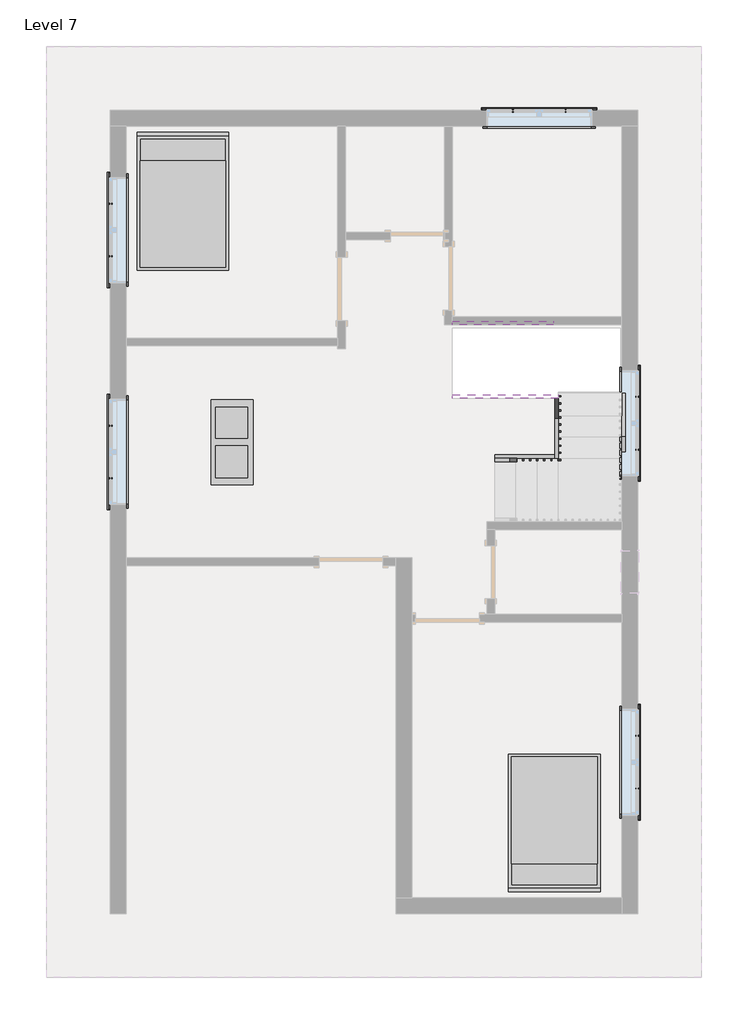
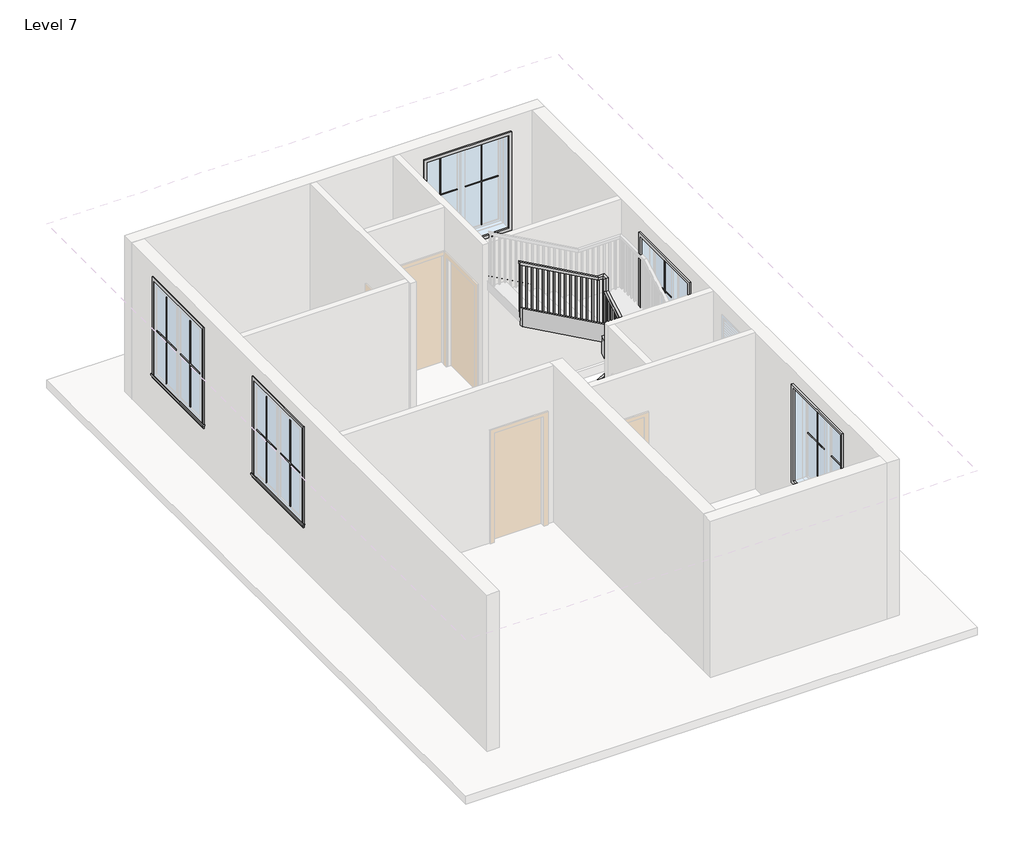
# One storey, part 2 of 2: 21 proxies, 6 members, 2 furniture elements, 1 railing.
"""IFC4 building model written with IfcOpenShell, lengths in millimetres."""

from ifc_helpers import new_model, si_unit, frame, origin, place, context, project, spatial, polyline, outline, extrude, faceted_brep, transform, mapped, element, save
from components import muntin_pattern_2x2_muntin_pattern_2x2_f6a80940, muntin_pattern_2x2_muntin_pattern_2x2_09b00a1c, trim_window_exterior_flat_with_sill_698ed857, trim_window_interior_flat_picture_frame_92551a5e, coffee_table_with_brass_mullions_11320_coffee_table_with_5962bef7, bed_17739_bed_17739_15c61121

model = new_model("IFC4")

# Units and contexts
model_context = context("Model", 3, world=origin())
ifc_project = project(units=[si_unit("LENGTHUNIT", "METRE", prefix="MILLI")], contexts=[model_context])

# Site, building, storey
site = spatial("IfcSite", under=ifc_project)
building = spatial("IfcBuilding", under=site)
storey = spatial("IfcBuildingStorey", under=building, Name="Level 7", Elevation=16002.0)

# Proxies
placement = place(None, origin())
muntin_pattern_2x2_muntin_pattern_2x2_shape = muntin_pattern_2x2_muntin_pattern_2x2_f6a80940(model_context)
element("IfcBuildingElementProxy", 1, Name="Muntin Pattern_2x2 : Muntin Pattern_2x2", ObjectType="Muntin Pattern_2x2 : Muntin Pattern_2x2", at=placement, inside=storey, context=model_context, shape_type="MappedRepresentation", body=[
    mapped(muntin_pattern_2x2_muntin_pattern_2x2_shape, transform((-4589.1575206, 441.8004493, 16986.25), x_axis=(0.0, 1.0, 0.0), y_axis=(-1.0, 0.0, 0.0), z_axis=(0.0, 0.0, 1.0))),
])
element("IfcBuildingElementProxy", 2, Name="Muntin Pattern_2x2 : Muntin Pattern_2x2", ObjectType="Muntin Pattern_2x2 : Muntin Pattern_2x2", at=placement, inside=storey, context=model_context, shape_type="MappedRepresentation", body=[
    mapped(muntin_pattern_2x2_muntin_pattern_2x2_shape, transform((-4589.1575206, 3632.6754493, 16986.25), x_axis=(0.0, 1.0, 0.0), y_axis=(-1.0, 0.0, 0.0), z_axis=(0.0, 0.0, 1.0))),
])
element("IfcBuildingElementProxy", 3, Name="Muntin Pattern_2x2 : Muntin Pattern_2x2", ObjectType="Muntin Pattern_2x2 : Muntin Pattern_2x2", at=placement, inside=storey, context=model_context, shape_type="MappedRepresentation", body=[
    mapped(muntin_pattern_2x2_muntin_pattern_2x2_shape, transform((1197.2799794, 5726.5879493, 16986.25), x_axis=(1.0, 0.0, 0.0), y_axis=(0.0, 1.0, 0.0), z_axis=(0.0, 0.0, 1.0))),
])
element("IfcBuildingElementProxy", 4, Name="Muntin Pattern_2x2 : Muntin Pattern_2x2", ObjectType="Muntin Pattern_2x2 : Muntin Pattern_2x2", at=placement, inside=storey, context=model_context, shape_type="MappedRepresentation", body=[
    mapped(muntin_pattern_2x2_muntin_pattern_2x2_shape, transform((2986.3924794, 1613.3754493, 16986.25), x_axis=(0.0, -1.0, 0.0), y_axis=(1.0, 0.0, 0.0), z_axis=(0.0, 0.0, 1.0))),
])
element("IfcBuildingElementProxy", 5, Name="Muntin Pattern_2x2 : Muntin Pattern_2x2", ObjectType="Muntin Pattern_2x2 : Muntin Pattern_2x2", at=placement, inside=storey, context=model_context, shape_type="MappedRepresentation", body=[
    mapped(muntin_pattern_2x2_muntin_pattern_2x2_shape, transform((2986.3924794, -3260.2495507, 16986.25), x_axis=(0.0, -1.0, 0.0), y_axis=(1.0, 0.0, 0.0), z_axis=(0.0, 0.0, 1.0))),
])
muntin_pattern_2x2_muntin_pattern_2x2_2_shape = muntin_pattern_2x2_muntin_pattern_2x2_09b00a1c(model_context)
element("IfcBuildingElementProxy", 6, Name="Muntin Pattern_2x2 : Muntin Pattern_2x2", ObjectType="Muntin Pattern_2x2 : Muntin Pattern_2x2", at=placement, inside=storey, context=model_context, shape_type="MappedRepresentation", body=[
    mapped(muntin_pattern_2x2_muntin_pattern_2x2_2_shape, transform((-4589.1575206, 1200.6254493, 16986.25), x_axis=(0.0, -1.0, 0.0), y_axis=(1.0, 0.0, 0.0), z_axis=(0.0, 0.0, 1.0))),
])
element("IfcBuildingElementProxy", 7, Name="Muntin Pattern_2x2 : Muntin Pattern_2x2", ObjectType="Muntin Pattern_2x2 : Muntin Pattern_2x2", at=placement, inside=storey, context=model_context, shape_type="MappedRepresentation", body=[
    mapped(muntin_pattern_2x2_muntin_pattern_2x2_2_shape, transform((-4589.1575206, 4391.5004493, 16986.25), x_axis=(0.0, -1.0, 0.0), y_axis=(1.0, 0.0, 0.0), z_axis=(0.0, 0.0, 1.0))),
])
element("IfcBuildingElementProxy", 8, Name="Muntin Pattern_2x2 : Muntin Pattern_2x2", ObjectType="Muntin Pattern_2x2 : Muntin Pattern_2x2", at=placement, inside=storey, context=model_context, shape_type="MappedRepresentation", body=[
    mapped(muntin_pattern_2x2_muntin_pattern_2x2_2_shape, transform((1956.1049794, 5726.5879493, 16986.25), x_axis=(-1.0, 0.0, 0.0), y_axis=(0.0, -1.0, 0.0), z_axis=(0.0, 0.0, 1.0))),
])
element("IfcBuildingElementProxy", 9, Name="Muntin Pattern_2x2 : Muntin Pattern_2x2", ObjectType="Muntin Pattern_2x2 : Muntin Pattern_2x2", at=placement, inside=storey, context=model_context, shape_type="MappedRepresentation", body=[
    mapped(muntin_pattern_2x2_muntin_pattern_2x2_2_shape, transform((2986.3924794, 854.5504493, 16986.25), x_axis=(0.0, 1.0, 0.0), y_axis=(-1.0, 0.0, 0.0), z_axis=(0.0, 0.0, 1.0))),
])
element("IfcBuildingElementProxy", 10, Name="Muntin Pattern_2x2 : Muntin Pattern_2x2", ObjectType="Muntin Pattern_2x2 : Muntin Pattern_2x2", at=placement, inside=storey, context=model_context, shape_type="MappedRepresentation", body=[
    mapped(muntin_pattern_2x2_muntin_pattern_2x2_2_shape, transform((2986.3924794, -4019.0745507, 16986.25), x_axis=(0.0, 1.0, 0.0), y_axis=(-1.0, 0.0, 0.0), z_axis=(0.0, 0.0, 1.0))),
])
trim_window_exterior_flat_with_sill_shape = trim_window_exterior_flat_with_sill_698ed857(model_context)
element("IfcBuildingElementProxy", 11, Name="Trim-Window-Exterior-Flat : with Sill", ObjectType="Trim-Window-Exterior-Flat : with Sill", at=placement, inside=storey, context=model_context, shape_type="MappedRepresentation", body=[
    mapped(trim_window_exterior_flat_with_sill_shape, transform((-4598.6825206, 821.2129493, 18745.2), x_axis=(0.0, -1.0, 0.0), y_axis=(0.0, 0.0, 1.0), z_axis=(-1.0, 0.0, 0.0))),
])
element("IfcBuildingElementProxy", 12, Name="Trim-Window-Exterior-Flat : with Sill", ObjectType="Trim-Window-Exterior-Flat : with Sill", at=placement, inside=storey, context=model_context, shape_type="MappedRepresentation", body=[
    mapped(trim_window_exterior_flat_with_sill_shape, transform((-4598.6825206, 4012.0879493, 18745.2), x_axis=(0.0, -1.0, 0.0), y_axis=(0.0, 0.0, 1.0), z_axis=(-1.0, 0.0, 0.0))),
])
element("IfcBuildingElementProxy", 13, Name="Trim-Window-Exterior-Flat : with Sill", ObjectType="Trim-Window-Exterior-Flat : with Sill", at=placement, inside=storey, context=model_context, shape_type="MappedRepresentation", body=[
    mapped(trim_window_exterior_flat_with_sill_shape, transform((1576.6924794, 5736.1129493, 18745.2), x_axis=(-1.0, 0.0, 0.0), y_axis=(0.0, 0.0, 1.0), z_axis=(0.0, 1.0, 0.0))),
])
element("IfcBuildingElementProxy", 14, Name="Trim-Window-Exterior-Flat : with Sill", ObjectType="Trim-Window-Exterior-Flat : with Sill", at=placement, inside=storey, context=model_context, shape_type="MappedRepresentation", body=[
    mapped(trim_window_exterior_flat_with_sill_shape, transform((2995.9174794, 1233.9629493, 18745.2), x_axis=(0.0, 1.0, 0.0), y_axis=(0.0, 0.0, 1.0), z_axis=(1.0, 0.0, 0.0))),
])
element("IfcBuildingElementProxy", 15, Name="Trim-Window-Exterior-Flat : with Sill", ObjectType="Trim-Window-Exterior-Flat : with Sill", at=placement, inside=storey, context=model_context, shape_type="MappedRepresentation", body=[
    mapped(trim_window_exterior_flat_with_sill_shape, transform((2995.9174794, -3639.6620507, 18745.2), x_axis=(0.0, 1.0, 0.0), y_axis=(0.0, 0.0, 1.0), z_axis=(1.0, 0.0, 0.0))),
])
trim_window_interior_flat_picture_frame_shape = trim_window_interior_flat_picture_frame_92551a5e(model_context)
element("IfcBuildingElementProxy", 16, Name="Trim-Window-Interior-Flat : Picture Frame", ObjectType="Trim-Window-Interior-Flat : Picture Frame", at=placement, inside=storey, context=model_context, shape_type="MappedRepresentation", body=[
    mapped(trim_window_interior_flat_picture_frame_shape, transform((-4370.0825206, 821.2129493, 18745.2), x_axis=(0.0, 1.0, 0.0), y_axis=(0.0, 0.0, 1.0), z_axis=(1.0, 0.0, 0.0))),
])
element("IfcBuildingElementProxy", 17, Name="Trim-Window-Interior-Flat : Picture Frame", ObjectType="Trim-Window-Interior-Flat : Picture Frame", at=placement, inside=storey, context=model_context, shape_type="MappedRepresentation", body=[
    mapped(trim_window_interior_flat_picture_frame_shape, transform((-4370.0825206, 4012.0879493, 18745.2), x_axis=(0.0, 1.0, 0.0), y_axis=(0.0, 0.0, 1.0), z_axis=(1.0, 0.0, 0.0))),
])
element("IfcBuildingElementProxy", 18, Name="Trim-Window-Interior-Flat : Picture Frame", ObjectType="Trim-Window-Interior-Flat : Picture Frame", at=placement, inside=storey, context=model_context, shape_type="MappedRepresentation", body=[
    mapped(trim_window_interior_flat_picture_frame_shape, transform((1576.6924794, 5507.5129493, 18745.2), x_axis=(1.0, 0.0, 0.0), y_axis=(0.0, 0.0, 1.0), z_axis=(0.0, -1.0, 0.0))),
])
element("IfcBuildingElementProxy", 19, Name="Trim-Window-Interior-Flat : Picture Frame", ObjectType="Trim-Window-Interior-Flat : Picture Frame", at=placement, inside=storey, context=model_context, shape_type="MappedRepresentation", body=[
    mapped(trim_window_interior_flat_picture_frame_shape, transform((2767.3174794, 1233.9629493, 18745.2), x_axis=(0.0, -1.0, 0.0), y_axis=(0.0, 0.0, 1.0), z_axis=(-1.0, 0.0, 0.0))),
])
element("IfcBuildingElementProxy", 20, Name="Trim-Window-Interior-Flat : Picture Frame", ObjectType="Trim-Window-Interior-Flat : Picture Frame", at=placement, inside=storey, context=model_context, shape_type="MappedRepresentation", body=[
    mapped(trim_window_interior_flat_picture_frame_shape, transform((2767.3174794, -3639.6620507, 18745.2), x_axis=(0.0, -1.0, 0.0), y_axis=(0.0, 0.0, 1.0), z_axis=(-1.0, 0.0, 0.0))),
])
coffee_table_with_brass_mullions_11320_coffee_table_with_shape = coffee_table_with_brass_mullions_11320_coffee_table_with_5962bef7(model_context)
element("IfcBuildingElementProxy", 21, Name="coffee_table_with_brass_mullions_11320 : coffee_table_with_brass_mullions_11320", ObjectType="coffee_table_with_brass_mullions_11320 : coffee_table_with_brass_mullions_11320", at=placement, inside=storey, context=model_context, shape_type="MappedRepresentation", body=[
    mapped(coffee_table_with_brass_mullions_11320_coffee_table_with_shape, transform((-2412.0418112, 1596.9678033, 16002.0), x_axis=(0.0, 1.0, 0.0), y_axis=(-1.0, 0.0, 0.0), z_axis=(0.0, 0.0, 1.0))),
])

# Furniture
bed_17739_bed_17739_shape = bed_17739_bed_17739_15c61121(model_context)
element("IfcFurniture", 22, ObjectType="Bed_17739 : Bed_17739", at=placement, inside=storey, context=model_context, shape_type="MappedRepresentation", body=[
    mapped(bed_17739_bed_17739_shape, transform((-3550.9325206, 4402.6129493, 16002.0), x_axis=(1.0, 0.0, 0.0), y_axis=(0.0, 1.0, 0.0), z_axis=(0.0, 0.0, 1.0))),
])
element("IfcFurniture", 23, ObjectType="Bed_17739 : Bed_17739", at=placement, inside=storey, context=model_context, shape_type="MappedRepresentation", body=[
    mapped(bed_17739_bed_17739_shape, transform((1795.7674794, -4487.3870507, 16002.0), x_axis=(-1.0, 0.0, 0.0), y_axis=(0.0, -1.0, 0.0), z_axis=(0.0, 0.0, 1.0))),
])

# Members
element("IfcMember", 24, ObjectType="Stringer - 2\" Width", at=placement, inside=storey, context=model_context, shape_type="SweptSolid", body=[
    extrude(outline(polyline([(16209.5983948, 938.5174794), (16002.0, 938.5174794), (16002.0, 1192.4619822), (16340.6974984, 1802.1174794), (16689.3761726, 1802.1174794), (16209.5983948, 938.5174794)])), frame((0.0, 732.3129493, 0.0), z_axis=(0.0, 1.0, 0.0), x_axis=(0.0, 0.0, 1.0)), (0.0, 0.0, 1.0), 50.8),
])
element("IfcMember", 25, ObjectType="Stringer - 2\" Width", at=placement, inside=storey, context=model_context, shape_type="SweptSolid", body=[
    extrude(outline(polyline([(732.3129493, 16538.253054), (732.3129493, 16886.9317281), (1595.9129493, 17366.7095059), (1595.9129493, 17018.0308318), (732.3129493, 16538.253054)])), frame((1802.1174794, 0.0, 0.0), z_axis=(1.0, 0.0, 0.0), x_axis=(0.0, 1.0, 0.0)), (0.0, 0.0, 1.0), 50.8),
])
element("IfcMember", 26, ObjectType="Stringer - 2\" Width", at=placement, inside=storey, context=model_context, shape_type="SweptSolid", body=[
    extrude(outline(polyline([(17215.5863873, 1852.9174794), (17564.2650614, 1852.9174794), (18410.9317281, 328.9174794), (18062.253054, 328.9174794), (17215.5863873, 1852.9174794)])), frame((0.0, 1595.9129493, 0.0), z_axis=(0.0, 1.0, 0.0), x_axis=(0.0, 0.0, 1.0)), (0.0, 0.0, 1.0), 50.8),
])
element("IfcMember", 27, ObjectType="Stringer - 2\" Width", at=placement, inside=storey, context=model_context, shape_type="SweptSolid", body=[
    extrude(outline(polyline([(16209.5983948, 938.5174794), (16002.0, 938.5174794), (16002.0, 1192.4619822), (16378.9317281, 1870.9390928), (16378.9317281, 1243.3174794), (16209.5983948, 938.5174794)])), frame((0.0, -232.8870507, 0.0), z_axis=(0.0, 1.0, 0.0), x_axis=(0.0, 0.0, 1.0)), (0.0, 0.0, 1.0), 50.8),
])
element("IfcMember", 28, ObjectType="Stringer - 2\" Width", at=placement, inside=storey, context=model_context, shape_type="SweptSolid", body=[
    extrude(outline(polyline([(714.2913359, 16876.9197207), (1037.1129493, 17056.2650614), (1664.7345627, 17056.2650614), (1341.9129493, 16876.9197207), (714.2913359, 16876.9197207)])), frame((2767.3174794, 0.0, 0.0), z_axis=(1.0, 0.0, 0.0), x_axis=(0.0, 1.0, 0.0)), (0.0, 0.0, 1.0), 50.8),
])
element("IfcMember", 29, ObjectType="Stringer - 2\" Width", at=placement, inside=storey, context=model_context, shape_type="SweptSolid", body=[
    extrude(outline(polyline([(17603.6419429, 1782.0390928), (18410.9317281, 328.9174794), (18062.253054, 328.9174794), (17603.6419429, 1154.4174794), (17603.6419429, 1782.0390928)])), frame((0.0, 2650.0129493, 0.0), z_axis=(0.0, 1.0, 0.0), x_axis=(0.0, 0.0, 1.0)), (0.0, 0.0, 1.0), 50.8),
])

# Railing
element("IfcRailing", 30, ObjectType="Handrail - Rectangular", at=placement, inside=storey, context=model_context, shape_type="SolidModel", body=[
    faceted_brep([(938.5174794, 732.3129493, 17085.7333333), (938.5174794, 732.3129493, 17027.620221), (938.5174794, 681.5129493, 17027.620221), (938.5174794, 681.5129493, 17085.7333333), (1776.7174794, 732.3129493, 17551.4), (1827.5174794, 732.3129493, 17521.5091099), (1827.5174794, 681.5129493, 17521.5091099), (1776.7174794, 681.5129493, 17551.4), (1776.7174794, 732.3129493, 17805.4), (1827.5174794, 732.3129493, 17754.6), (1827.5174794, 681.5129493, 17754.6), (1776.7174794, 681.5129493, 17805.4), (1852.9174794, 732.3129493, 17805.4), (1852.9174794, 732.3129493, 17754.6), (1903.7174794, 681.5129493, 17754.6), (1903.7174794, 681.5129493, 17805.4), (1852.9174794, 808.5129493, 17805.4), (1852.9174794, 821.6765516, 17754.6), (1903.7174794, 821.6765516, 17754.6), (1903.7174794, 808.5129493, 17805.4), (1852.9174794, 1570.5129493, 18228.7333333), (1852.9174794, 1621.3129493, 18198.8424432), (1903.7174794, 1621.3129493, 18198.8424432), (1903.7174794, 1570.5129493, 18228.7333333), (1852.9174794, 1570.5129493, 18482.7333333), (1852.9174794, 1621.3129493, 18431.9333333), (1903.7174794, 1621.3129493, 18431.9333333), (1903.7174794, 1570.5129493, 18482.7333333), (1852.9174794, 1646.7129493, 18482.7333333), (1852.9174794, 1646.7129493, 18431.9333333), (1903.7174794, 1697.5129493, 18431.9333333), (1903.7174794, 1697.5129493, 18482.7333333), (1776.7174794, 1646.7129493, 18482.7333333), (1763.5538772, 1646.7129493, 18431.9333333), (1763.5538772, 1697.5129493, 18431.9333333), (1776.7174794, 1697.5129493, 18482.7333333), (328.9174794, 1646.7129493, 19287.0666667), (328.9174794, 1697.5129493, 19287.0666667), (328.9174794, 1697.5129493, 19228.9535543), (328.9174794, 1646.7129493, 19228.9535543)], [[[0, 1, 2, 3]], [[1, 0, 4, 5]], [[2, 1, 5, 6]], [[3, 2, 6, 7]], [[0, 3, 7, 4]], [[5, 4, 8, 9]], [[6, 5, 9, 10]], [[7, 6, 10, 11]], [[4, 7, 11, 8]], [[9, 8, 12, 13]], [[10, 9, 13, 14]], [[11, 10, 14, 15]], [[8, 11, 15, 12]], [[13, 12, 16, 17]], [[14, 13, 17, 18]], [[15, 14, 18, 19]], [[12, 15, 19, 16]], [[17, 16, 20, 21]], [[18, 17, 21, 22]], [[19, 18, 22, 23]], [[16, 19, 23, 20]], [[21, 20, 24, 25]], [[22, 21, 25, 26]], [[23, 22, 26, 27]], [[20, 23, 27, 24]], [[25, 24, 28, 29]], [[26, 25, 29, 30]], [[27, 26, 30, 31]], [[24, 27, 31, 28]], [[29, 28, 32, 33]], [[30, 29, 33, 34]], [[31, 30, 34, 35]], [[28, 31, 35, 32]], [[36, 37, 38, 39]], [[33, 32, 36, 39]], [[34, 33, 39, 38]], [[35, 34, 38, 37]], [[32, 35, 37, 36]]]),
    extrude(outline(polyline([(19220.1341099, 344.7924794), (18203.3333333, 344.7924794), (18203.3333333, 363.8424794), (19209.5507765, 363.8424794), (19220.1341099, 344.7924794)])), frame((0.0, 1662.5879493, 0.0), z_axis=(0.0, 1.0, 0.0), x_axis=(0.0, 0.0, 1.0)), (0.0, 0.0, 1.0), 19.05),
    extrude(outline(polyline([(19163.6896654, 446.3924794), (18203.3333333, 446.3924794), (18203.3333333, 465.4424794), (19153.1063321, 465.4424794), (19163.6896654, 446.3924794)])), frame((0.0, 1662.5879493, 0.0), z_axis=(0.0, 1.0, 0.0), x_axis=(0.0, 0.0, 1.0)), (0.0, 0.0, 1.0), 19.05),
    extrude(outline(polyline([(19107.245221, 547.9924794), (18203.3333333, 547.9924794), (18203.3333333, 567.0424794), (19096.6618876, 567.0424794), (19107.245221, 547.9924794)])), frame((0.0, 1662.5879493, 0.0), z_axis=(0.0, 1.0, 0.0), x_axis=(0.0, 0.0, 1.0)), (0.0, 0.0, 1.0), 19.05),
    extrude(outline(polyline([(19050.8007765, 649.5924794), (18034.0, 649.5924794), (18034.0, 668.6424794), (19040.2174432, 668.6424794), (19050.8007765, 649.5924794)])), frame((0.0, 1662.5879493, 0.0), z_axis=(0.0, 1.0, 0.0), x_axis=(0.0, 0.0, 1.0)), (0.0, 0.0, 1.0), 19.05),
    extrude(outline(polyline([(18994.3563321, 751.1924794), (18034.0, 751.1924794), (18034.0, 770.2424794), (18983.7729988, 770.2424794), (18994.3563321, 751.1924794)])), frame((0.0, 1662.5879493, 0.0), z_axis=(0.0, 1.0, 0.0), x_axis=(0.0, 0.0, 1.0)), (0.0, 0.0, 1.0), 19.05),
    extrude(outline(polyline([(18937.9118876, 852.7924794), (18034.0, 852.7924794), (18034.0, 871.8424794), (18927.3285543, 871.8424794), (18937.9118876, 852.7924794)])), frame((0.0, 1662.5879493, 0.0), z_axis=(0.0, 1.0, 0.0), x_axis=(0.0, 0.0, 1.0)), (0.0, 0.0, 1.0), 19.05),
    extrude(outline(polyline([(18881.4674432, 954.3924794), (17864.6666667, 954.3924794), (17864.6666667, 973.4424794), (18870.8841099, 973.4424794), (18881.4674432, 954.3924794)])), frame((0.0, 1662.5879493, 0.0), z_axis=(0.0, 1.0, 0.0), x_axis=(0.0, 0.0, 1.0)), (0.0, 0.0, 1.0), 19.05),
    extrude(outline(polyline([(18825.0229988, 1055.9924794), (17864.6666667, 1055.9924794), (17864.6666667, 1075.0424794), (18814.4396654, 1075.0424794), (18825.0229988, 1055.9924794)])), frame((0.0, 1662.5879493, 0.0), z_axis=(0.0, 1.0, 0.0), x_axis=(0.0, 0.0, 1.0)), (0.0, 0.0, 1.0), 19.05),
    extrude(outline(polyline([(18768.5785543, 1157.5924794), (17864.6666667, 1157.5924794), (17864.6666667, 1176.6424794), (18757.995221, 1176.6424794), (18768.5785543, 1157.5924794)])), frame((0.0, 1662.5879493, 0.0), z_axis=(0.0, 1.0, 0.0), x_axis=(0.0, 0.0, 1.0)), (0.0, 0.0, 1.0), 19.05),
    extrude(outline(polyline([(18712.1341099, 1259.1924794), (17695.3333333, 1259.1924794), (17695.3333333, 1278.2424794), (18701.5507765, 1278.2424794), (18712.1341099, 1259.1924794)])), frame((0.0, 1662.5879493, 0.0), z_axis=(0.0, 1.0, 0.0), x_axis=(0.0, 0.0, 1.0)), (0.0, 0.0, 1.0), 19.05),
    extrude(outline(polyline([(18655.6896654, 1360.7924794), (17695.3333333, 1360.7924794), (17695.3333333, 1379.8424794), (18645.1063321, 1379.8424794), (18655.6896654, 1360.7924794)])), frame((0.0, 1662.5879493, 0.0), z_axis=(0.0, 1.0, 0.0), x_axis=(0.0, 0.0, 1.0)), (0.0, 0.0, 1.0), 19.05),
    extrude(outline(polyline([(18599.245221, 1462.3924794), (17695.3333333, 1462.3924794), (17695.3333333, 1481.4424794), (18588.6618876, 1481.4424794), (18599.245221, 1462.3924794)])), frame((0.0, 1662.5879493, 0.0), z_axis=(0.0, 1.0, 0.0), x_axis=(0.0, 0.0, 1.0)), (0.0, 0.0, 1.0), 19.05),
    extrude(outline(polyline([(18542.8007765, 1563.9924794), (17526.0, 1563.9924794), (17526.0, 1583.0424794), (18532.2174432, 1583.0424794), (18542.8007765, 1563.9924794)])), frame((0.0, 1662.5879493, 0.0), z_axis=(0.0, 1.0, 0.0), x_axis=(0.0, 0.0, 1.0)), (0.0, 0.0, 1.0), 19.05),
    extrude(outline(polyline([(18486.3563321, 1665.5924794), (17526.0, 1665.5924794), (17526.0, 1684.6424794), (18475.7729988, 1684.6424794), (18486.3563321, 1665.5924794)])), frame((0.0, 1662.5879493, 0.0), z_axis=(0.0, 1.0, 0.0), x_axis=(0.0, 0.0, 1.0)), (0.0, 0.0, 1.0), 19.05),
    extrude(outline(polyline([(18429.9118876, 1767.1924794), (17526.0, 1767.1924794), (17526.0, 1786.2424794), (18419.3285543, 1786.2424794), (18429.9118876, 1767.1924794)])), frame((0.0, 1662.5879493, 0.0), z_axis=(0.0, 1.0, 0.0), x_axis=(0.0, 0.0, 1.0)), (0.0, 0.0, 1.0), 19.05),
    extrude(outline(polyline([(1868.7924794, 1611.7879493), (1868.7924794, 1630.8379493), (1887.8424794, 1630.8379493), (1887.8424794, 1611.7879493), (1868.7924794, 1611.7879493)])), frame((0.0, 0.0, 17187.3333333), z_axis=(0.0, 0.0, 1.0), x_axis=(1.0, 0.0, 0.0)), (0.0, 0.0, 1.0), 1244.6),
    extrude(outline(polyline([(1529.2379493, 18147.6896654), (1529.2379493, 17187.3333333), (1510.1879493, 17187.3333333), (1510.1879493, 18137.1063321), (1529.2379493, 18147.6896654)])), frame((1868.7924794, 0.0, 0.0), z_axis=(1.0, 0.0, 0.0), x_axis=(0.0, 1.0, 0.0)), (0.0, 0.0, 1.0), 19.05),
    extrude(outline(polyline([(1427.6379493, 18091.245221), (1427.6379493, 17187.3333333), (1408.5879493, 17187.3333333), (1408.5879493, 18080.6618876), (1427.6379493, 18091.245221)])), frame((1868.7924794, 0.0, 0.0), z_axis=(1.0, 0.0, 0.0), x_axis=(0.0, 1.0, 0.0)), (0.0, 0.0, 1.0), 19.05),
    extrude(outline(polyline([(1326.0379493, 18034.8007765), (1326.0379493, 17018.0), (1306.9879493, 17018.0), (1306.9879493, 18024.2174432), (1326.0379493, 18034.8007765)])), frame((1868.7924794, 0.0, 0.0), z_axis=(1.0, 0.0, 0.0), x_axis=(0.0, 1.0, 0.0)), (0.0, 0.0, 1.0), 19.05),
    extrude(outline(polyline([(1224.4379493, 17978.3563321), (1224.4379493, 17018.0), (1205.3879493, 17018.0), (1205.3879493, 17967.7729988), (1224.4379493, 17978.3563321)])), frame((1868.7924794, 0.0, 0.0), z_axis=(1.0, 0.0, 0.0), x_axis=(0.0, 1.0, 0.0)), (0.0, 0.0, 1.0), 19.05),
    extrude(outline(polyline([(1122.8379493, 17921.9118876), (1122.8379493, 17018.0), (1103.7879493, 17018.0), (1103.7879493, 17911.3285543), (1122.8379493, 17921.9118876)])), frame((1868.7924794, 0.0, 0.0), z_axis=(1.0, 0.0, 0.0), x_axis=(0.0, 1.0, 0.0)), (0.0, 0.0, 1.0), 19.05),
    extrude(outline(polyline([(1021.2379493, 17865.4674432), (1021.2379493, 16848.6666667), (1002.1879493, 16848.6666667), (1002.1879493, 17854.8841099), (1021.2379493, 17865.4674432)])), frame((1868.7924794, 0.0, 0.0), z_axis=(1.0, 0.0, 0.0), x_axis=(0.0, 1.0, 0.0)), (0.0, 0.0, 1.0), 19.05),
    extrude(outline(polyline([(919.6379493, 17809.0229988), (919.6379493, 16848.6666667), (900.5879493, 16848.6666667), (900.5879493, 17798.4396654), (919.6379493, 17809.0229988)])), frame((1868.7924794, 0.0, 0.0), z_axis=(1.0, 0.0, 0.0), x_axis=(0.0, 1.0, 0.0)), (0.0, 0.0, 1.0), 19.05),
    extrude(outline(polyline([(818.0379493, 17752.5785543), (818.0379493, 16848.6666667), (798.9879493, 16848.6666667), (798.9879493, 17741.995221), (818.0379493, 17752.5785543)])), frame((1868.7924794, 0.0, 0.0), z_axis=(1.0, 0.0, 0.0), x_axis=(0.0, 1.0, 0.0)), (0.0, 0.0, 1.0), 19.05),
    extrude(outline(polyline([(1843.3924794, 716.4379493), (1862.4424794, 716.4379493), (1862.4424794, 697.3879493), (1843.3924794, 697.3879493), (1843.3924794, 716.4379493)])), frame((0.0, 0.0, 16679.3333333), z_axis=(0.0, 0.0, 1.0), x_axis=(1.0, 0.0, 0.0)), (0.0, 0.0, 1.0), 1075.2666667),
    extrude(outline(polyline([(17473.8841099, 1741.7924794), (16510.0, 1741.7924794), (16510.0, 1760.8424794), (17484.4674432, 1760.8424794), (17473.8841099, 1741.7924794)])), frame((0.0, 697.3879493, 0.0), z_axis=(0.0, 1.0, 0.0), x_axis=(0.0, 0.0, 1.0)), (0.0, 0.0, 1.0), 19.05),
    extrude(outline(polyline([(17417.4396654, 1640.1924794), (16510.0, 1640.1924794), (16510.0, 1659.2424794), (17428.0229988, 1659.2424794), (17417.4396654, 1640.1924794)])), frame((0.0, 697.3879493, 0.0), z_axis=(0.0, 1.0, 0.0), x_axis=(0.0, 0.0, 1.0)), (0.0, 0.0, 1.0), 19.05),
    extrude(outline(polyline([(17360.995221, 1538.5924794), (16510.0, 1538.5924794), (16510.0, 1557.6424794), (17371.5785543, 1557.6424794), (17360.995221, 1538.5924794)])), frame((0.0, 697.3879493, 0.0), z_axis=(0.0, 1.0, 0.0), x_axis=(0.0, 0.0, 1.0)), (0.0, 0.0, 1.0), 19.05),
    extrude(outline(polyline([(17304.5507765, 1436.9924794), (16340.6666667, 1436.9924794), (16340.6666667, 1456.0424794), (17315.1341099, 1456.0424794), (17304.5507765, 1436.9924794)])), frame((0.0, 697.3879493, 0.0), z_axis=(0.0, 1.0, 0.0), x_axis=(0.0, 0.0, 1.0)), (0.0, 0.0, 1.0), 19.05),
    extrude(outline(polyline([(17248.1063321, 1335.3924794), (16340.6666667, 1335.3924794), (16340.6666667, 1354.4424794), (17258.6896654, 1354.4424794), (17248.1063321, 1335.3924794)])), frame((0.0, 697.3879493, 0.0), z_axis=(0.0, 1.0, 0.0), x_axis=(0.0, 0.0, 1.0)), (0.0, 0.0, 1.0), 19.05),
    extrude(outline(polyline([(17191.6618876, 1233.7924794), (16340.6666667, 1233.7924794), (16340.6666667, 1252.8424794), (17202.245221, 1252.8424794), (17191.6618876, 1233.7924794)])), frame((0.0, 697.3879493, 0.0), z_axis=(0.0, 1.0, 0.0), x_axis=(0.0, 0.0, 1.0)), (0.0, 0.0, 1.0), 19.05),
    extrude(outline(polyline([(17135.2174432, 1132.1924794), (16171.3333333, 1132.1924794), (16171.3333333, 1151.2424794), (17145.8007765, 1151.2424794), (17135.2174432, 1132.1924794)])), frame((0.0, 697.3879493, 0.0), z_axis=(0.0, 1.0, 0.0), x_axis=(0.0, 0.0, 1.0)), (0.0, 0.0, 1.0), 19.05),
    extrude(outline(polyline([(17078.7729988, 1030.5924794), (16171.3333333, 1030.5924794), (16171.3333333, 1049.6424794), (17089.3563321, 1049.6424794), (17078.7729988, 1030.5924794)])), frame((0.0, 697.3879493, 0.0), z_axis=(0.0, 1.0, 0.0), x_axis=(0.0, 0.0, 1.0)), (0.0, 0.0, 1.0), 19.05),
    extrude(outline(polyline([(1868.7924794, 1662.5879493), (1868.7924794, 1681.6379493), (1887.8424794, 1681.6379493), (1887.8424794, 1662.5879493), (1868.7924794, 1662.5879493)])), frame((0.0, 0.0, 17356.6666667), z_axis=(0.0, 0.0, 1.0), x_axis=(1.0, 0.0, 0.0)), (0.0, 0.0, 1.0), 1075.2666667),
    extrude(outline(polyline([(1868.7924794, 716.4379493), (1887.8424794, 716.4379493), (1887.8424794, 697.3879493), (1868.7924794, 697.3879493), (1868.7924794, 716.4379493)])), frame((0.0, 0.0, 16679.3333333), z_axis=(0.0, 0.0, 1.0), x_axis=(1.0, 0.0, 0.0)), (0.0, 0.0, 1.0), 1075.2666667),
    extrude(outline(polyline([(19228.9535543, 328.9174794), (18203.3333333, 328.9174794), (18203.3333333, 347.9674794), (19218.370221, 347.9674794), (19228.9535543, 328.9174794)])), frame((0.0, 1662.5879493, 0.0), z_axis=(0.0, 1.0, 0.0), x_axis=(0.0, 0.0, 1.0)), (0.0, 0.0, 1.0), 19.05),
    extrude(outline(polyline([(17027.620221, 938.5174794), (16171.3333333, 938.5174794), (16171.3333333, 957.5674794), (17038.2035543, 957.5674794), (17027.620221, 938.5174794)])), frame((0.0, 697.3879493, 0.0), z_axis=(0.0, 1.0, 0.0), x_axis=(0.0, 0.0, 1.0)), (0.0, 0.0, 1.0), 19.05),
])

save(model, "model.ifc")

# Revit data of these elements
# Type "Muntin Pattern_2x2 : Muntin Pattern_2x2"
#   Width [instance default] = 4' - 0"
#   Thickness = 0' - 0 1/2"
#   Height [instance default] = 4' - 0"
#   Distance = 0' - 0 3/4"
#   Interior Material [instance default] = none
#   Exterior Material [instance default] = none
#   Default Elevation = 0
# Type "Trim-Window-Exterior-Flat : with Sill"
#   Trim Width = 0' - 2 1/4"
#   Trim Thickness_Picture Frame = 0' - 1 1/4"
#   Trim Thickness_with Sill = 0' - 0 3/4"
#   Sill Thickness = 0' - 1 1/4"
#   Opening Width [instance default] = 2' - 0"
#   Opening Height [instance default] = 3' - 0"
#   Default Elevation = 4' - 0"
#   Sill = yes
#   Picture Frame = no
#   Trim Material [instance default] = none
# Type "Trim-Window-Interior-Flat : Picture Frame"
#   Trim Thickness_Picture Frame = 0' - 1 1/4"
#   Trim Width = 0' - 2 1/4"
#   Trim Thickness_with Sill = 0' - 0 3/4"
#   Sill Thickness = 0' - 1 1/4"
#   Opening Width [instance default] = 2' - 0"
#   Opening Height [instance default] = 3' - 0"
#   Default Elevation = 4' - 0"
#   Sill = no
#   Picture Frame = yes
#   Trim Material [instance default] = none
# Type "coffee_table_with_brass_mullions_11320 : coffee_table_with_brass_mullions_11320"
#   Default Elevation = 0
# Type "Bed_17739 : Bed_17739"
#   Default Elevation = 0
# Type "Handrail - Rectangular"
#   Assembly Code = "C2010400"
#   built-in parameter 1008612 = 0.0416667 (stored number, unit not read)
#   built-in parameter 1008611 = 0.0416667 (stored number, unit not read)
#   built-in parameter 1008609 = 0.333333 (stored number, unit not read)
#   built-in parameter 1008604 = 0.166667 (stored number, unit not read)
#   built-in parameter 1008603 = 0.166667 (stored number, unit not read)
#   Railing Height = 3' - 0"
#   built-in parameter 1008630 = 2
#   built-in parameter 1008610 = 2
#   built-in parameter 1008618 = Baluster - Square : 3/4"
# Elements 1, 2, 3, 4, 5, 6, 7, 8, 9, 10 (IfcBuildingElementProxy, "Muntin Pattern_2x2 : Muntin Pattern_2x2")
#   Width = 2' - 0 5/8"
#   Height = 5' - 6 1/2"
#   Interior Material = Wood - Stained
#   Exterior Material = Clad - White
#   Phase Created = New Construction
#   Materials on its faces: "Clad - White", "Wood - Stained"
# Elements 11, 12, 13, 14, 15 (IfcBuildingElementProxy, "Trim-Window-Exterior-Flat : with Sill")
#   Opening Width = 5' - 0"
#   Opening Height = 6' - 0"
#   Trim Material = Clad - White
#   Phase Created = New Construction
#   Materials on its faces: "Clad - White"
# Elements 16, 17, 18, 19, 20 (IfcBuildingElementProxy, "Trim-Window-Interior-Flat : Picture Frame")
#   Opening Width = 5' - 0"
#   Opening Height = 6' - 0"
#   Trim Material = Wood - Stained
#   Phase Created = New Construction
#   Materials on its faces: "Wood - Stained"
# Element 21 (IfcBuildingElementProxy, "coffee_table_with_brass_mullions_11320 : coffee_table_with_brass_mullions_11320")
#   Phase Created = New Construction
#   Materials on its faces: "Default Wall", "TABLE", "Glass", "Default"
# Elements 22, 23 (IfcFurniture, "Bed_17739 : Bed_17739")
#   Phase Created = New Construction
#   Materials on its faces: "legs", "sheets", "bed frame", "Blanket"
# Elements 24, 25, 26, 27, 28, 29 (IfcMember, "Stringer - 2\" Width")
#   Phase Created = New Construction
# Element 30 (IfcRailing, "Handrail - Rectangular")
#   Phase Created = New Construction
# Materials
#   "Clad - White": class "Wood", colour RGB 242 242 238, transparency 0, Cost = 0
#   "Wood - Stained": class "Wood", colour RGB 224 178 126, transparency 0, Cost = 0
#   "Default Wall": colour RGB 128 128 128, transparency 0, Cost = 0
#   "TABLE": class "Generic", colour RGB 120 120 120, transparency 0, Cost = 0
#   "Glass": class "Glass", colour RGB 0 128 192, transparency 0.75, Description = "Soda Lime Glass", Cost = 0
#   "Default": colour RGB 127 127 127, transparency 0, Cost = 0
#   "legs": colour RGB 90 73 37, transparency 0, Cost = 0
#   "sheets": colour RGB 200 195 176, transparency 0, Cost = 0
#   "bed frame": colour RGB 90 73 37, transparency 0, Cost = 0
#   "Blanket": class "System", colour RGB 59 0 1, transparency 0, Cost = 0
